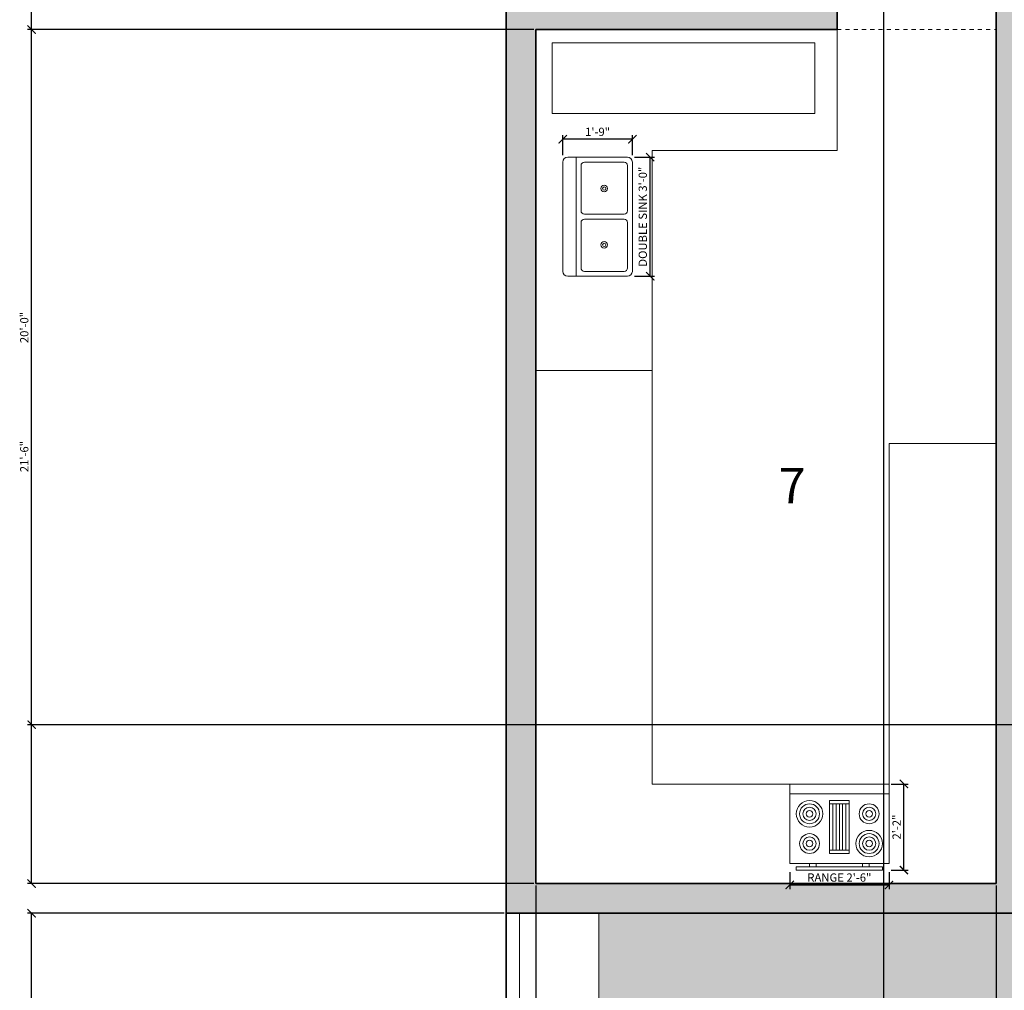
# Model space of a CAD drawing. Units: inches. Extents: x 3122 to 5933, y 1474 to 2995.
# Tile 4 of 12: x 4918 to 5215, y 2032 to 2326. Entities that reach past the tile are written whole.
import ezdxf

# ---------------------------------------------------------------- set-up
doc = ezdxf.new("R2010")
doc.units = ezdxf.units.IN
doc.linetypes.add('JIS_02_1.2', pattern=[2.5, 1.25, -1.25])
for name, color, linetype, lineweight in [('A-ANNO-DIMS', 2, 'Continuous', 18), ('A-AREA-IDEN', 7, 'Continuous', 20), ('A-EQPM', 9, 'Continuous', 20), ('A-FLOR-CASE', 8, 'Continuous', 18), ('A-FLOR-FIXT', 9, 'Continuous', 18), ('A-FLOR-OVHD', 8, 'JIS_02_1.2', 18), ('A-WALL', 7, 'Continuous', 35), ('A-WALL-PATT', 7, 'Continuous', 13), ('C-PROP', 7, 'Continuous', 25), ('L-PLNT', 3, 'Continuous', 18), ('L-PLNT-PATT', 94, 'Continuous', 13)]:
    doc.layers.add(name, color=color, linetype=linetype, lineweight=lineweight)
doc.styles.get("Standard").update_dxf_attribs({"font": 'arial.ttf'})
doc.dimstyles.new('ISO-25', dxfattribs={"dimtxt": 2.5, "dimasz": 2.5, "dimexe": 1.25, "dimexo": 0.625, "dimtad": 1, "dimdec": 0, "dimlunit": 3, "dimtxsty": 'Standard', "dimblk": 'ARCHTICK', "dimcen": 2.5, "dimadec": 0, "dimazin": 0, "dimtfac": 1, "dimtdec": 0, "dimtmove": 0, "dimatfit": 3, "dimfxl": 1, "dimarcsym": 0})

# ---------------------------------------------------------------- blocks, each defined once
blk = doc.blocks.new('Sink-double - 36 in top')
for p, q in [((-18, -4), (18, -4)), ((-0.75, -18.5), (-0.75, -6.5)), ((0.75, -6.5), (0.75, -18.5))]:
    blk.add_line(p, q)
for points in [[(-16.5, 0), (16.5, 0)], [(-18, -19.5), (-18, -1.5)], [(18, -1.5), (18, -19.5)], [(-15.5, -5.5), (-1.75, -5.5)], [(1.75, -5.5), (15.5, -5.5)], [(-16.5, -18.5), (-16.5, -6.5)], [(16.5, -6.5), (16.5, -18.5)], [(-1.75, -19.5), (-15.5, -19.5)], [(15.5, -19.5), (1.75, -19.5)], [(16.5, -21), (-16.5, -21)]]:
    blk.add_lwpolyline(points)
for centre, radius in [((-8.5, -12.5), 1), ((8.5, -12.5), 1), ((-8.5, -12.5), 0.5), ((8.5, -12.5), 0.5)]:
    blk.add_circle(centre, radius)
for centre, radius, start, end in [((-16.5, -1.5), 1.5, 90, 180), ((16.5, -1.5), 1.5, 0, 90), ((-15.5, -6.5), 1, 90, 180), ((-1.75, -6.5), 1, 0, 90), ((1.75, -6.5), 1, 90, 180), ((15.5, -6.5), 1, 0, 90), ((-16.5, -19.5), 1.5, 180, 270), ((-15.5, -18.5), 1, 180, 270), ((-1.75, -18.5), 1, 270, 0), ((1.75, -18.5), 1, 180, 270), ((15.5, -18.5), 1, 270, 0), ((16.5, -19.5), 1.5, 270, 0)]:
    blk.add_arc(centre, radius, start, end)
blk = doc.blocks.new('Range-Oven - 30 in top')
for p, q in [((0, -3), (30, -3)), ((12, -6), (18, -6)), ((13, -20), (13, -6)), ((14, -6), (14, -20)), ((15, -20), (15, -6)), ((16, -6), (16, -20)), ((17, -20), (17, -6)), ((18, -20), (12, -20)), ((6, -24), (6, -25)), ((8, -25), (8, -24)), ((22, -25), (22, -24)), ((24, -24), (24, -25))]:
    blk.add_line(p, q)
for points in [[(0, -24), (0, 0), (30, 0), (30, -24)], [(12, -21), (12, -5), (18, -5), (18, -21)], [(2, -26), (2, -25), (28, -25), (28, -26)]]:
    blk.add_lwpolyline(points, close=True)
for centre, radius in [((6, -9), 4), ((6, -9), 3), ((6, -9), 2), ((6, -9), 1), ((24, -9), 3), ((24, -9), 2), ((24, -9), 1), ((24, -18), 4), ((6, -18), 3), ((6, -18), 2), ((6, -18), 1), ((24, -18), 3), ((24, -18), 2), ((24, -18), 1)]:
    blk.add_circle(centre, radius)
blk = doc.blocks.new('_ArchTick')
at = {"color": 0, "linetype": 'ByBlock', "const_width": 0.15}
blk.add_lwpolyline([(-0.5, -0.5), (0.5, 0.5)], dxfattribs=at)
blk = doc.blocks.new('*D84')
at = {"layer": 'A-ANNO-DIMS', "color": 0, "lineweight": -2, "transparency": 16777216}
for p, q in [((5103.71, 2284.16), (5109.74, 2284.16)), ((5108.49, 2248.16), (5108.49, 2284.16)), ((5103.71, 2248.16), (5109.74, 2248.16))]:
    blk.add_line(p, q, dxfattribs=at)
at = {"layer": 'Defpoints', "color": 0, "transparency": 16777216}
for p in [(5103.09, 2284.16), (5108.49, 2284.16), (5103.09, 2248.16)]:
    blk.add_point(p, dxfattribs=at)
at = {"layer": 'A-ANNO-DIMS', "color": 0, "lineweight": -2, "transparency": 16777216, "xscale": 2.5, "yscale": 2.5, "zscale": 2.5}
for p, rotation in [((5108.49, 2284.16), 90), ((5108.49, 2248.16), 270)]:
    blk.add_blockref('_ArchTick', p, dxfattribs=dict(at, rotation=rotation))
at = {"layer": 'A-ANNO-DIMS', "color": 0, "transparency": 16777216, "insert": (5106.57, 2266.16), "char_height": 2.5, "attachment_point": 5, "rotation": 90}
blk.add_mtext('DOUBLE SINK 3\'-0"', dxfattribs=at)
blk = doc.blocks.new('*D85')
at = {"layer": 'A-ANNO-DIMS', "color": 0, "lineweight": -2, "transparency": 16777216}
for p, q in [((5082.09, 2284.79), (5082.09, 2290.81)), ((5103.09, 2284.79), (5103.09, 2290.81)), ((5103.09, 2289.56), (5082.09, 2289.56))]:
    blk.add_line(p, q, dxfattribs=at)
at = {"layer": 'Defpoints', "color": 0, "transparency": 16777216}
for p in [(5082.09, 2289.56), (5082.09, 2284.16), (5103.09, 2284.16)]:
    blk.add_point(p, dxfattribs=at)
at = {"layer": 'A-ANNO-DIMS', "color": 0, "lineweight": -2, "transparency": 16777216, "xscale": 2.5, "yscale": 2.5, "zscale": 2.5, "rotation": 180}
blk.add_blockref('_ArchTick', (5082.09, 2289.56), dxfattribs=at)
at = {"layer": 'A-ANNO-DIMS', "color": 0, "lineweight": -2, "transparency": 16777216, "xscale": 2.5, "yscale": 2.5, "zscale": 2.5}
blk.add_blockref('_ArchTick', (5103.09, 2289.56), dxfattribs=at)
at = {"layer": 'A-ANNO-DIMS', "color": 0, "transparency": 16777216, "insert": (5092.59, 2291.47), "char_height": 2.5, "attachment_point": 5}
blk.add_mtext('1\'-9"', dxfattribs=at)
blk = doc.blocks.new('*D86')
at = {"layer": 'A-ANNO-DIMS', "color": 0, "lineweight": -2, "transparency": 16777216}
for p, q in [((5150.63, 2068.15), (5150.63, 2063.02)), ((5180.63, 2068.15), (5180.63, 2063.02)), ((5150.63, 2064.27), (5180.63, 2064.27))]:
    blk.add_line(p, q, dxfattribs=at)
at = {"layer": 'Defpoints', "color": 0, "transparency": 16777216}
for p in [(5150.63, 2068.77), (5180.63, 2068.77), (5180.63, 2064.27)]:
    blk.add_point(p, dxfattribs=at)
at = {"layer": 'A-ANNO-DIMS', "color": 0, "lineweight": -2, "transparency": 16777216, "xscale": 2.5, "yscale": 2.5, "zscale": 2.5, "rotation": 180}
blk.add_blockref('_ArchTick', (5150.63, 2064.27), dxfattribs=at)
at = {"layer": 'A-ANNO-DIMS', "color": 0, "lineweight": -2, "transparency": 16777216, "xscale": 2.5, "yscale": 2.5, "zscale": 2.5}
blk.add_blockref('_ArchTick', (5180.63, 2064.27), dxfattribs=at)
at = {"layer": 'A-ANNO-DIMS', "color": 0, "transparency": 16777216, "insert": (5165.63, 2066.19), "char_height": 2.5, "attachment_point": 5}
blk.add_mtext('RANGE 2\'-6"', dxfattribs=at)
blk = doc.blocks.new('*D87')
at = {"layer": 'A-ANNO-DIMS', "color": 0, "lineweight": -2, "transparency": 16777216}
for p, q in [((5181.25, 2094.77), (5186.38, 2094.77)), ((5185.13, 2068.77), (5185.13, 2094.77)), ((5181.25, 2068.77), (5186.38, 2068.77))]:
    blk.add_line(p, q, dxfattribs=at)
at = {"layer": 'Defpoints', "color": 0, "transparency": 16777216}
for p in [(5180.63, 2094.77), (5185.13, 2094.77), (5180.63, 2068.77)]:
    blk.add_point(p, dxfattribs=at)
at = {"layer": 'A-ANNO-DIMS', "color": 0, "lineweight": -2, "transparency": 16777216, "xscale": 2.5, "yscale": 2.5, "zscale": 2.5}
for p, rotation in [((5185.13, 2094.77), 90), ((5185.13, 2068.77), 270)]:
    blk.add_blockref('_ArchTick', p, dxfattribs=dict(at, rotation=rotation))
at = {"layer": 'A-ANNO-DIMS', "color": 0, "transparency": 16777216, "insert": (5183.25, 2081.77), "char_height": 2.5, "attachment_point": 5, "rotation": 90}
blk.add_mtext('2\'-2"', dxfattribs=at)
blk = doc.blocks.new('*D94')
at = {"layer": 'A-ANNO-DIMS', "color": 0, "lineweight": -2, "transparency": 16777216}
for p, q in [((5064.96, 1916.52), (5064.96, 2990.75)), ((5064.96, 2989.5), (5487.87, 2989.5)), ((5487.87, 1916.52), (5487.87, 2990.75))]:
    blk.add_line(p, q, dxfattribs=at)
at = {"layer": 'Defpoints', "color": 0, "transparency": 16777216}
for p in [(5487.87, 2989.5), (5064.96, 1915.9), (5487.87, 1915.9)]:
    blk.add_point(p, dxfattribs=at)
at = {"layer": 'A-ANNO-DIMS', "color": 0, "lineweight": -2, "transparency": 16777216, "xscale": 2.5, "yscale": 2.5, "zscale": 2.5, "rotation": 180}
blk.add_blockref('_ArchTick', (5064.96, 2989.5), dxfattribs=at)
at = {"layer": 'A-ANNO-DIMS', "color": 0, "lineweight": -2, "transparency": 16777216, "xscale": 2.5, "yscale": 2.5, "zscale": 2.5}
blk.add_blockref('_ArchTick', (5487.87, 2989.5), dxfattribs=at)
at = {"layer": 'A-ANNO-DIMS', "color": 0, "transparency": 16777216, "insert": (5276.42, 2991.41), "char_height": 2.5, "attachment_point": 5}
blk.add_mtext('35\'-3"', dxfattribs=at)
blk = doc.blocks.new('*D97')
at = {"layer": 'A-ANNO-DIMS', "color": 0, "lineweight": -2, "transparency": 16777216}
for p, q in [((5064.34, 2055.71), (4920.36, 2055.71)), ((4921.61, 1915.9), (4921.61, 2055.71)), ((5064.34, 1915.9), (4920.36, 1915.9))]:
    blk.add_line(p, q, dxfattribs=at)
at = {"layer": 'Defpoints', "color": 0, "transparency": 16777216}
for p in [(4921.61, 2055.71), (5064.96, 2055.71), (5064.96, 1915.9)]:
    blk.add_point(p, dxfattribs=at)
at = {"layer": 'A-ANNO-DIMS', "color": 0, "lineweight": -2, "transparency": 16777216, "xscale": 2.5, "yscale": 2.5, "zscale": 2.5}
for p, rotation in [((4921.61, 2055.71), 90), ((4921.61, 1915.9), 270)]:
    blk.add_blockref('_ArchTick', p, dxfattribs=dict(at, rotation=rotation))
at = {"layer": 'A-ANNO-DIMS', "color": 0, "transparency": 16777216, "insert": (4919.71, 1985.8), "char_height": 2.5, "attachment_point": 5, "rotation": 90}
blk.add_mtext('11\'-8"', dxfattribs=at)
blk = doc.blocks.new('*D98')
at = {"layer": 'A-ANNO-DIMS', "color": 0, "lineweight": -2, "transparency": 16777216}
for p, q in [((5073.34, 2322.69), (4920.36, 2322.69)), ((4921.61, 2064.71), (4921.61, 2322.69)), ((5073.34, 2064.71), (4920.36, 2064.71))]:
    blk.add_line(p, q, dxfattribs=at)
at = {"layer": 'Defpoints', "color": 0, "transparency": 16777216}
for p in [(4921.61, 2322.69), (5073.96, 2322.69), (5073.96, 2064.71)]:
    blk.add_point(p, dxfattribs=at)
at = {"layer": 'A-ANNO-DIMS', "color": 0, "lineweight": -2, "transparency": 16777216, "xscale": 2.5, "yscale": 2.5, "zscale": 2.5}
for p, rotation in [((4921.61, 2322.69), 90), ((4921.61, 2064.71), 270)]:
    blk.add_blockref('_ArchTick', p, dxfattribs=dict(at, rotation=rotation))
at = {"layer": 'A-ANNO-DIMS', "color": 0, "transparency": 16777216, "insert": (4919.71, 2193.7), "char_height": 2.5, "attachment_point": 5, "rotation": 90}
blk.add_mtext('21\'-6"', dxfattribs=at)
blk = doc.blocks.new('*D102')
at = {"layer": 'A-ANNO-DIMS', "color": 0, "lineweight": -2, "transparency": 16777216}
for p, q in [((5073.96, 2064.08), (5073.96, 1792.93)), ((5212.96, 2064.08), (5212.96, 1792.93)), ((5073.96, 1794.18), (5212.96, 1794.18))]:
    blk.add_line(p, q, dxfattribs=at)
at = {"layer": 'Defpoints', "color": 0, "transparency": 16777216}
for p in [(5073.96, 2064.71), (5212.96, 2064.71), (5212.96, 1794.18)]:
    blk.add_point(p, dxfattribs=at)
at = {"layer": 'A-ANNO-DIMS', "color": 0, "lineweight": -2, "transparency": 16777216, "xscale": 2.5, "yscale": 2.5, "zscale": 2.5, "rotation": 180}
blk.add_blockref('_ArchTick', (5073.96, 1794.18), dxfattribs=at)
at = {"layer": 'A-ANNO-DIMS', "color": 0, "lineweight": -2, "transparency": 16777216, "xscale": 2.5, "yscale": 2.5, "zscale": 2.5}
blk.add_blockref('_ArchTick', (5212.96, 1794.18), dxfattribs=at)
at = {"layer": 'A-ANNO-DIMS', "color": 0, "transparency": 16777216, "insert": (5143.46, 1796.06), "char_height": 2.5, "attachment_point": 5}
blk.add_mtext('11\'-7"', dxfattribs=at)
blk = doc.blocks.new('*D104')
at = {"layer": 'A-ANNO-DIMS', "color": 0, "lineweight": -2, "transparency": 16777216}
for p, q in [((5427.24, 2352.69), (4920.36, 2352.69)), ((4921.61, 2112.69), (4921.61, 2352.69)), ((5427.24, 2112.69), (4920.36, 2112.69))]:
    blk.add_line(p, q, dxfattribs=at)
at = {"layer": 'Defpoints', "color": 0, "transparency": 16777216}
for p in [(4921.61, 2352.69), (5427.87, 2352.69), (5427.87, 2112.69)]:
    blk.add_point(p, dxfattribs=at)
at = {"layer": 'A-ANNO-DIMS', "color": 0, "lineweight": -2, "transparency": 16777216, "xscale": 2.5, "yscale": 2.5, "zscale": 2.5}
for p, rotation in [((4921.61, 2352.69), 90), ((4921.61, 2112.69), 270)]:
    blk.add_blockref('_ArchTick', p, dxfattribs=dict(at, rotation=rotation))
at = {"layer": 'A-ANNO-DIMS', "color": 0, "transparency": 16777216, "insert": (4919.71, 2232.69), "char_height": 2.5, "attachment_point": 5, "rotation": 90}
blk.add_mtext('20\'-0"', dxfattribs=at)
blk = doc.blocks.new('*D108')
at = {"layer": 'A-ANNO-DIMS', "color": 0, "lineweight": -2, "transparency": 16777216}
for p, q in [((5178.96, 2643.06), (5178.96, 1792.93)), ((5358.96, 2643.06), (5358.96, 1792.93)), ((5178.96, 1794.18), (5358.96, 1794.18))]:
    blk.add_line(p, q, dxfattribs=at)
at = {"layer": 'Defpoints', "color": 0, "transparency": 16777216}
for p in [(5178.96, 2643.69), (5358.96, 2643.69), (5358.96, 1794.18)]:
    blk.add_point(p, dxfattribs=at)
at = {"layer": 'A-ANNO-DIMS', "color": 0, "lineweight": -2, "transparency": 16777216, "xscale": 2.5, "yscale": 2.5, "zscale": 2.5, "rotation": 180}
blk.add_blockref('_ArchTick', (5178.96, 1794.18), dxfattribs=at)
at = {"layer": 'A-ANNO-DIMS', "color": 0, "lineweight": -2, "transparency": 16777216, "xscale": 2.5, "yscale": 2.5, "zscale": 2.5}
blk.add_blockref('_ArchTick', (5358.96, 1794.18), dxfattribs=at)
at = {"layer": 'A-ANNO-DIMS', "color": 0, "transparency": 16777216, "insert": (5268.96, 1796.08), "char_height": 2.5, "attachment_point": 5}
blk.add_mtext('15\'-0"', dxfattribs=at)

msp = doc.modelspace()

# ---------------------------------------------------------------- hatches: boundary and pattern name
at = {"layer": 'A-WALL-PATT'}
h = msp.add_hatch(color=256, dxfattribs=at)
h.dxf.hatch_style = 1
h.paths.add_polyline_path([(5073.96, 2454.69), (5101.59, 2454.69), (5101.59, 2459.69), (5101.59, 2463.69), (5073.96, 2463.69), (5073.96, 2634.69), (5169.96, 2634.69), (5364.96, 2634.69), (5364.96, 2643.69), (5364.96, 2667.06), (5358.96, 2667.06), (5358.96, 2643.69), (5178.96, 2643.69), (5178.96, 2655.69), (5169.96, 2655.69), (5169.96, 2643.69), (5073.96, 2643.69), (5073.96, 2745.9), (5124.13, 2745.9), (5124.13, 2754.9), (5073.96, 2754.9), (5073.96, 2866.9), (5169.96, 2866.9), (5169.96, 2818.9), (5169.96, 2812.9), (5169.96, 2754.9), (5154.13, 2754.9), (5154.13, 2745.9), (5169.96, 2745.9), (5169.96, 2691.69), (5178.96, 2691.69), (5178.96, 2812.9), (5178.96, 2818.9), (5178.96, 2875.9), (5064.96, 2875.9), (5064.96, 2055.71), (5217.96, 2055.71), (5217.96, 2464.19), (5212.96, 2464.19), (5212.96, 2463.69), (5148.19, 2463.69), (5148.19, 2459.69), (5148.19, 2454.69), (5158.96, 2454.69), (5158.96, 2450.72), (5156.04, 2450.72), (5156.04, 2447.72), (5158.96, 2447.72), (5158.96, 2425.1), (5164.96, 2425.1), (5164.96, 2447.72), (5167.71, 2447.72), (5167.71, 2450.72), (5164.96, 2450.72), (5164.96, 2454.69), (5212.96, 2454.69), (5212.96, 2064.71), (5073.96, 2064.71), (5073.96, 2322.69), (5158.96, 2322.69), (5164.96, 2322.69), (5164.96, 2328.69), (5158.96, 2328.69), (5073.96, 2328.69)])
at = {"layer": 'L-PLNT-PATT'}
h = msp.add_hatch(dxfattribs=at)
h.set_pattern_fill('GRASS', color=256, scale=0.1)
h.paths.add_polyline_path([(5463.87, 2047.66), (5427.87, 2047.66), (5217.96, 2047.66), (5217.96, 2055.71), (5092.96, 2055.71), (5092.96, 1919.9), (5463.87, 1919.9)])

# ---------------------------------------------------------------- linework, layer by layer
at = {"layer": 'A-FLOR-CASE'}
for p, q in [((5164.96, 2322.69), (5164.96, 2286.14)), ((5164.96, 2286.14), (5109.12, 2286.14)), ((5109.12, 2286.14), (5109.12, 2094.77)), ((5109.12, 2219.73), (5073.96, 2219.73)), ((5180.63, 2094.77), (5180.63, 2197.67)), ((5180.63, 2197.67), (5212.96, 2197.67)), ((5109.12, 2094.77), (5180.63, 2094.77))]:
    msp.add_line(p, q, dxfattribs=at)
msp.add_lwpolyline([(5078.91, 2318.65), (5158.19, 2318.65), (5158.19, 2297.34), (5078.91, 2297.34)], close=True, dxfattribs=at)
at = {"layer": 'A-FLOR-OVHD'}
msp.add_line((5164.96, 2322.69), (5212.96, 2322.69), dxfattribs=at)
at = {"layer": 'A-WALL'}
for p, q in [((5212.96, 2454.69), (5212.96, 2064.71)), ((5164.96, 2328.69), (5164.96, 2322.69)), ((5073.96, 2322.69), (5158.96, 2322.69)), ((5073.96, 2322.69), (5073.96, 2064.71)), ((5158.96, 2322.69), (5164.96, 2322.69)), ((5212.96, 2064.71), (5073.96, 2064.71)), ((5217.96, 2055.71), (5064.96, 2055.71))]:
    msp.add_line(p, q, dxfattribs=at)
at = {"layer": 'C-PROP'}
msp.add_line((5064.96, 2875.9), (5064.96, 1915.9), dxfattribs=at)
at = {"layer": 'L-PLNT'}
for p, q in [((5068.96, 2055.71), (5068.96, 1919.9)), ((5092.96, 2055.71), (5092.96, 1919.9))]:
    msp.add_line(p, q, dxfattribs=at)

# ---------------------------------------------------------------- block references
at = {"layer": 'A-EQPM'}
msp.add_blockref('Range-Oven - 30 in top', (5150.63, 2094.77), dxfattribs=at)
at = {"layer": 'A-FLOR-FIXT', "rotation": 90}
msp.add_blockref('Sink-double - 36 in top', (5082.09, 2266.16), dxfattribs=at)

# ---------------------------------------------------------------- texts
at = {"layer": 'A-AREA-IDEN'}
msp.add_text('7', height=10.72, rotation=0.0333, dxfattribs=at).set_placement((5147.34, 2179.56))

# ---------------------------------------------------------------- dimensions: what is measured, and where the dimension line sits
at = {"layer": 'A-ANNO-DIMS'}
for base, p1, p2, picture, middle in [((5487.87, 2989.5), (5064.96, 1915.9), (5487.87, 1915.9), '*D94', (5276.42, 2991.41)), ((5358.96, 1794.18), (5178.96, 2643.69), (5358.96, 2643.69), '*D108', (5268.96, 1796.08)), ((5212.96, 1794.18), (5073.96, 2064.71), (5212.96, 2064.71), '*D102', (5143.46, 1796.06))]:
    dim = msp.add_linear_dim(base=base, p1=p1, p2=p2, dimstyle='ISO-25', override={"dimdec": 1, "dimlfac": 1, "dimrnd": 0, "dimzin": 1, "dimdsep": 46, "dimlunit": 4, "dimfrac": 2}, dxfattribs=at)
    dim.commit()
    dim.dimension.update_dxf_attribs({"geometry": picture, "text_midpoint": middle})
for base, p1, p2, angle, picture, middle in [((4921.61, 2352.69), (5427.87, 2112.69), (5427.87, 2352.69), 90, '*D104', (4919.71, 2232.69)), ((4921.61, 2322.69), (5073.96, 2064.71), (5073.96, 2322.69), 90, '*D98', (4919.71, 2193.7)), ((5082.09, 2289.56), (5103.09, 2284.16), (5082.09, 2284.16), 180, '*D85', (5092.59, 2291.47)), ((5185.13, 2094.77), (5180.63, 2068.77), (5180.63, 2094.77), 90, '*D87', (5183.25, 2081.77)), ((4921.61, 2055.71), (5064.96, 1915.9), (5064.96, 2055.71), 90, '*D97', (4919.71, 1985.8))]:
    dim = msp.add_linear_dim(base=base, p1=p1, p2=p2, angle=angle, dimstyle='ISO-25', override={"dimdec": 1, "dimlfac": 1, "dimrnd": 0, "dimzin": 1, "dimdsep": 46, "dimlunit": 4, "dimfrac": 2}, dxfattribs=at)
    dim.commit()
    dim.dimension.update_dxf_attribs({"geometry": picture, "text_midpoint": middle})
dim = msp.add_linear_dim(base=(5108.49, 2284.16), p1=(5103.09, 2248.16), p2=(5103.09, 2284.16), angle=90, text='DOUBLE SINK <>', dimstyle='ISO-25', override={"dimdec": 1, "dimlfac": 1, "dimrnd": 0, "dimzin": 1, "dimdsep": 46, "dimlunit": 4, "dimfrac": 2}, dxfattribs=at)
dim.commit()
dim.dimension.update_dxf_attribs({"geometry": '*D84', "text_midpoint": (5106.57, 2266.16)})
dim = msp.add_linear_dim(base=(5180.63, 2064.27), p1=(5150.63, 2068.77), p2=(5180.63, 2068.77), text='RANGE <>', dimstyle='ISO-25', override={"dimdec": 1, "dimlfac": 1, "dimrnd": 0, "dimzin": 1, "dimdsep": 46, "dimlunit": 4, "dimfrac": 2}, dxfattribs=at)
dim.commit()
dim.dimension.update_dxf_attribs({"geometry": '*D86', "text_midpoint": (5165.63, 2066.19)})

doc.saveas('drawing.dxf')
